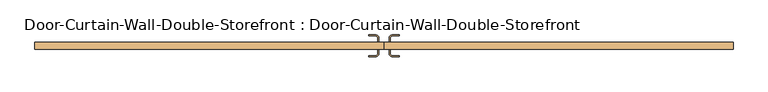
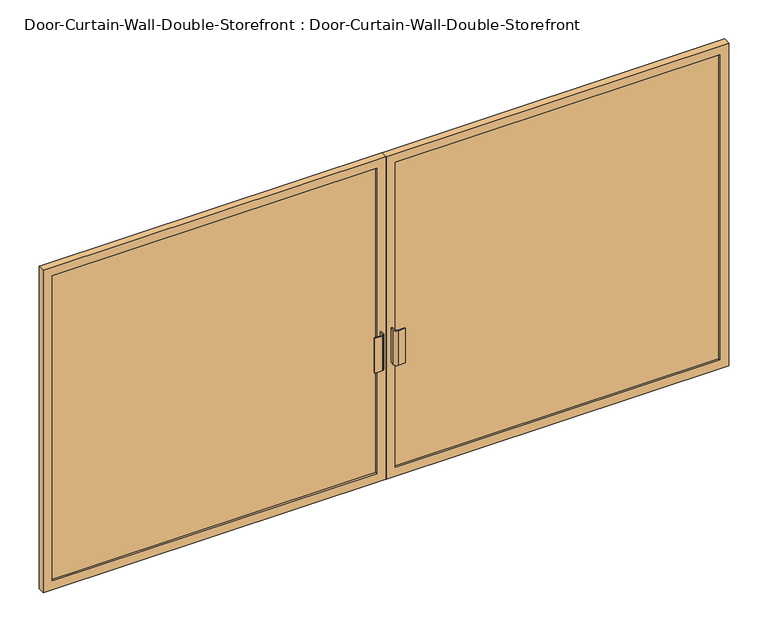
"""IFC4 building model written with IfcOpenShell, lengths in millimetres: door geometry, Door-Curtain-Wall-Double-Storefront : Door-Curtain-Wall-Double-Storefront."""

from ifc_helpers import new_model, si_unit, point, frame, frame_2d, origin, place, context, project, spatial, polyline, circle_curve, trimmed, segment, composite_curve, outline, extrude, source, transform, mapped, element, save


def door_curtain_wall_double_storefront_door_curtain_wall_double_6e8ba87c(model_context):
    return source(origin(), model_context, "Body", "SweptSolid", [
        extrude(outline(polyline([(2133.6, 0.7668501), (0.0, 0.7668501), (0.0, 2146.3), (2133.6, 2146.3), (2133.6, 0.7668501)]), holes=[polyline([(2076.45, 57.9168501), (2076.45, 2089.15), (57.15, 2089.15), (57.15, 57.9168501), (2076.45, 57.9168501)])]), frame((0.0, 12.7, 0.0), z_axis=(0.0, 1.0, 0.0), x_axis=(0.0, 0.0, 1.0)), (0.0, 0.0, 1.0), 44.45),
        extrude(outline(polyline([(2133.6, -0.8206499), (2133.6, -2146.3), (0.0, -2146.3), (0.0, -0.8206499), (2133.6, -0.8206499)]), holes=[polyline([(2076.45, -2089.15), (2076.45, -57.9706499), (57.15, -57.9706499), (57.15, -2089.15), (2076.45, -2089.15)])]), frame((0.0, 12.7, 0.0), z_axis=(0.0, 1.0, 0.0), x_axis=(0.0, 0.0, 1.0)), (0.0, 0.0, 1.0), 44.45),
        extrude(outline(polyline([(2089.15, 25.4), (57.9168501, 25.4), (57.9168501, 44.45), (2089.15, 44.45), (2089.15, 25.4)])), frame((0.0, 0.0, 57.15), z_axis=(0.0, 0.0, 1.0), x_axis=(1.0, 0.0, 0.0)), (0.0, 0.0, 1.0), 2019.3),
        extrude(outline(polyline([(-57.9706499, 25.4), (-2089.15, 25.4), (-2089.15, 44.45), (-57.9706499, 44.45), (-57.9706499, 25.4)])), frame((0.0, 0.0, 57.15), z_axis=(0.0, 0.0, 1.0), x_axis=(1.0, 0.0, 0.0)), (0.0, 0.0, 1.0), 2019.3),
        extrude(outline(composite_curve([segment(trimmed(circle_curve(frame_2d((-50.8268999, -12.7)), 19.05), [point((-31.7768999, -12.7))], [point((-50.8268999, -31.75))], False, "CARTESIAN"), True, "CONTINUOUS"), segment(polyline([(-50.8268999, -31.75), (-95.2768999, -31.75), (-95.2768999, -25.4), (-50.8268999, -25.4)]), True, "CONTINUOUS"), segment(trimmed(circle_curve(frame_2d((-50.8268999, -12.7)), 12.7), [point((-50.8268999, -25.4))], [point((-38.1268999, -12.7))], True, "CARTESIAN"), True, "CONTINUOUS"), segment(polyline([(-38.1268999, -12.7), (-38.1268999, 12.7), (-31.7768999, 12.7), (-31.7768999, -12.7)]), True, "CONTINUOUS")], self_intersect=False)), frame((0.0, 0.0, 762.0), z_axis=(0.0, 0.0, 1.0), x_axis=(1.0, 0.0, 0.0)), (0.0, 0.0, 1.0), 228.6),
        extrude(outline(composite_curve([segment(polyline([(31.7231001, -12.7), (31.7231001, 12.7), (38.0731001, 12.7), (38.0731001, -12.7)]), True, "CONTINUOUS"), segment(trimmed(circle_curve(frame_2d((50.7731001, -12.7)), 12.7), [point((38.0731001, -12.7))], [point((50.7731001, -25.4))], True, "CARTESIAN"), True, "CONTINUOUS"), segment(polyline([(50.7731001, -25.4), (95.2231001, -25.4), (95.2231001, -31.75), (50.7731001, -31.75)]), True, "CONTINUOUS"), segment(trimmed(circle_curve(frame_2d((50.7731001, -12.7)), 19.05), [point((50.7731001, -31.75))], [point((31.7231001, -12.7))], False, "CARTESIAN"), True, "CONTINUOUS")], self_intersect=False)), frame((0.0, 0.0, 762.0), z_axis=(0.0, 0.0, 1.0), x_axis=(1.0, 0.0, 0.0)), (0.0, 0.0, 1.0), 228.6),
        extrude(outline(composite_curve([segment(polyline([(-31.7768999, 82.55), (-31.7768999, 57.15), (-38.1268999, 57.15), (-38.1268999, 82.55)]), True, "CONTINUOUS"), segment(trimmed(circle_curve(frame_2d((-50.8268999, 82.55)), 12.7), [point((-38.1268999, 82.55))], [point((-50.8268999, 95.25))], True, "CARTESIAN"), True, "CONTINUOUS"), segment(polyline([(-50.8268999, 95.25), (-95.2768999, 95.25), (-95.2768999, 101.6), (-50.8268999, 101.6)]), True, "CONTINUOUS"), segment(trimmed(circle_curve(frame_2d((-50.8268999, 82.55)), 19.05), [point((-50.8268999, 101.6))], [point((-31.7768999, 82.55))], False, "CARTESIAN"), True, "CONTINUOUS")], self_intersect=False)), frame((0.0, 0.0, 762.0), z_axis=(0.0, 0.0, 1.0), x_axis=(1.0, 0.0, 0.0)), (0.0, 0.0, 1.0), 228.6),
        extrude(outline(composite_curve([segment(trimmed(circle_curve(frame_2d((50.7731001, 82.55)), 19.05), [point((31.7231001, 82.55))], [point((50.7731001, 101.6))], False, "CARTESIAN"), True, "CONTINUOUS"), segment(polyline([(50.7731001, 101.6), (95.2231001, 101.6), (95.2231001, 95.25), (50.7731001, 95.25)]), True, "CONTINUOUS"), segment(trimmed(circle_curve(frame_2d((50.7731001, 82.55)), 12.7), [point((50.7731001, 95.25))], [point((38.0731001, 82.55))], True, "CARTESIAN"), True, "CONTINUOUS"), segment(polyline([(38.0731001, 82.55), (38.0731001, 57.15), (31.7231001, 57.15), (31.7231001, 82.55)]), True, "CONTINUOUS")], self_intersect=False)), frame((0.0, 0.0, 762.0), z_axis=(0.0, 0.0, 1.0), x_axis=(1.0, 0.0, 0.0)), (0.0, 0.0, 1.0), 228.6),
    ])


if __name__ == "__main__":
    model = new_model("IFC4")
    model_context = context("Model", 3, world=origin())
    ifc_project = project(units=[si_unit("LENGTHUNIT", "METRE", prefix="MILLI")], contexts=[model_context])
    site = spatial("IfcSite", under=ifc_project)
    building = spatial("IfcBuilding", under=site)
    placement = place(None, origin())
    door_curtain_wall_double_storefront_door_curtain_wall_double_shape = door_curtain_wall_double_storefront_door_curtain_wall_double_6e8ba87c(model_context)
    element("IfcDoor", 1, ObjectType="Door-Curtain-Wall-Double-Storefront : Door-Curtain-Wall-Double-Storefront", at=placement, inside=building, context=model_context, shape_type="MappedRepresentation", body=[
        mapped(door_curtain_wall_double_storefront_door_curtain_wall_double_shape, transform((0.0, 0.0, 0.0), x_axis=(1.0, 0.0, 0.0), y_axis=(0.0, 1.0, 0.0), z_axis=(0.0, 0.0, 1.0))),
    ])
    save(model, "model.ifc")

# Revit data of these elements
# Type "Door-Curtain-Wall-Double-Storefront : Door-Curtain-Wall-Double-Storefront"
#   Type Mark = "14"
#   Construction Type Id = "opn-d46"
#   Assembly Code = "B2030100"
#   Analytic Construction = "Metal frame, double glass door"
#   Width [instance default] = 6' - 0"
#   Thermal Resistance (R) = 1.3794 (h·ft²·°F)/BTU
#   Swing Angle [instance default] = 90.00°
#   Panel Width [instance default] = 3' - 0"
#   Offset = 0' - 2 1/4"
#   Heat Transfer Coefficient (U) = 0.7250 BTU/(h·ft²·°F)
#   Define Thermal Properties by = 1
#   Function = 1
#   Frame Material = Aluminum
#   Door Handle Material = Aluminum
#   Glazing = Glass
#   Visual Light Transmittance = 0
#   Solar Heat Gain Coefficient = 0
# Element 1 (IfcDoor, "Door-Curtain-Wall-Double-Storefront : Door-Curtain-Wall-Double-Storefront")
#   Width = 14' - 1"
#   Panel Width = 7' - 0 1/2"
#   Materials on its faces: "Aluminum", "Glass"
# Materials
#   "Aluminum": class "Metal", colour RGB 247 247 247, transparency 0, Description = "Aluminum 6061", Cost = 0
#   "Glass": class "Glass", colour RGB 0 128 192, transparency 0.75, Description = "Soda Lime Glass", Cost = 0
